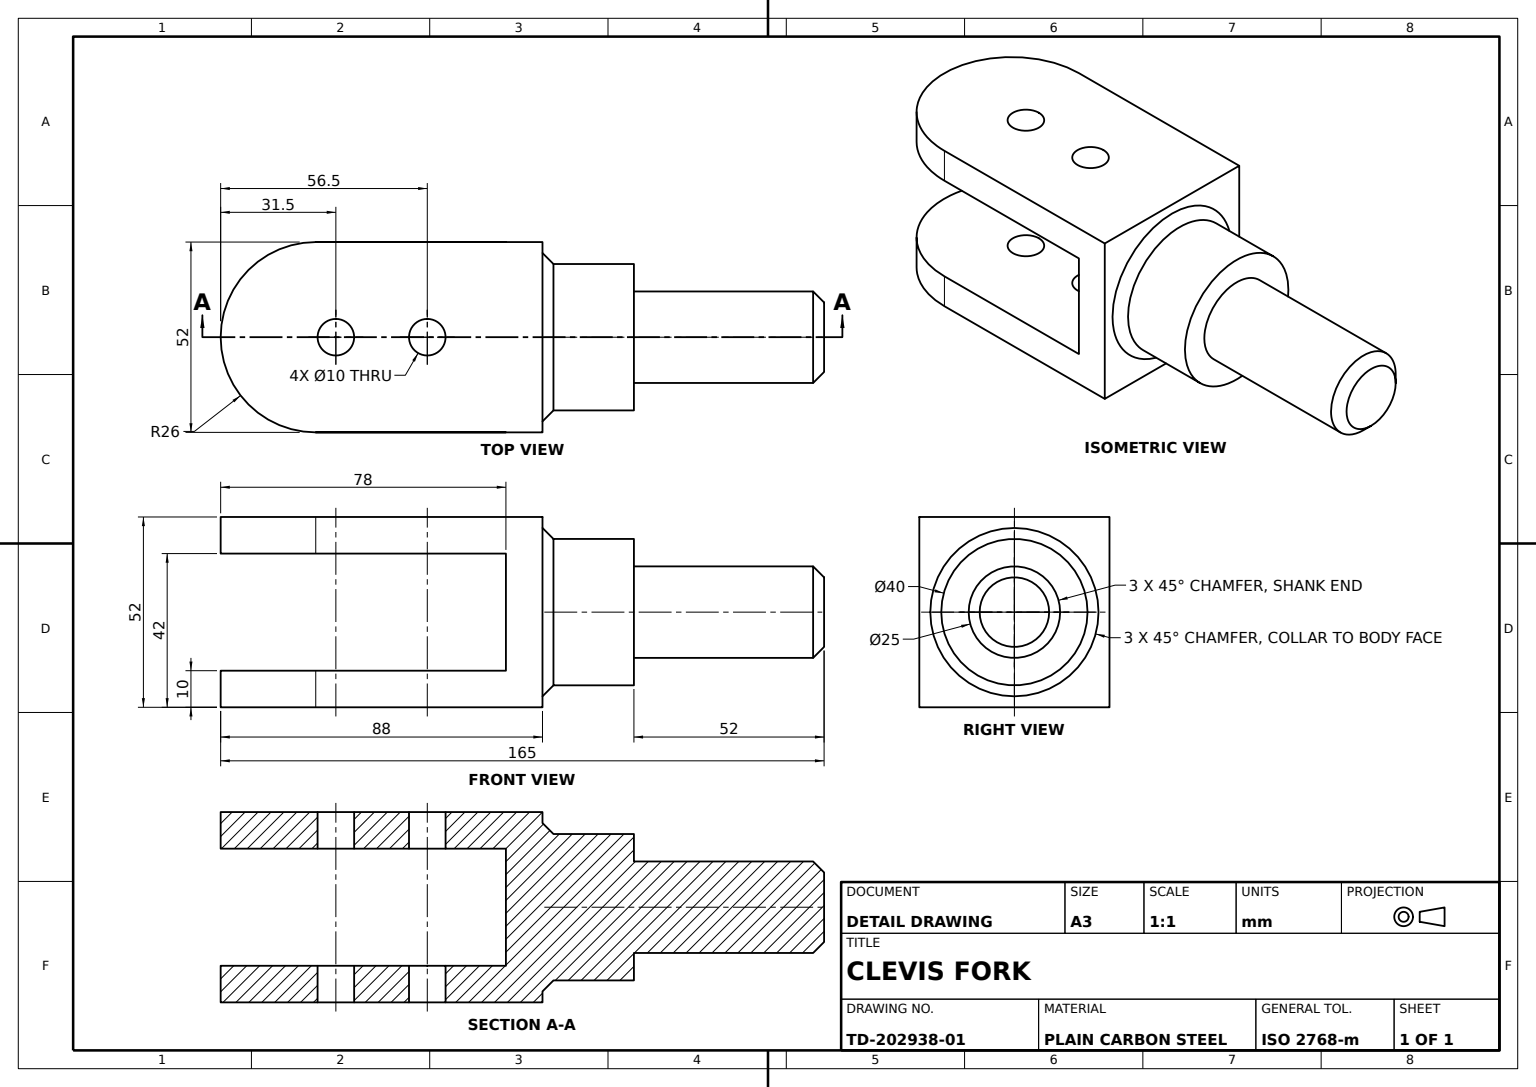
from build123d import *

# Parameters (mm, degrees)
CLEVIS_BODY_52MM_DEPTH          = 52
ARM_END_BOSS_1_DEPTH            = 10
ARM_START                       = -10
ARM_END_BOSS_2_DEPTH            = 10
FORK_START                      = -70
FORK_TRIM_CUT_DEPTH             = 70
FORK_SLOT_PROFILE_W             = 26
FORK_SLOT_PROFILE_H             = 52
FORK_SLOT_CUT_DEPTH             = 70
ARM_END_BOSS_3_DEPTH            = 10
ARM_END_BOSS_4_DEPTH            = 10
COLLAR_PROFILE_R                = 20
COLLAR_25MM_DEPTH               = 25
COLLAR_CHAMFER_3X45_SIZE        = 3
SHANK_PROFILE_R                 = 12.5
SHANK_52MM_DEPTH                = 52
SHANK_END_CHAMFER_3X45_SIZE     = 3
PIN_HOLES_PROFILE_R             = 5
PIN_HOLES_2X_THROUGH_ARMS_DEPTH = 52


with BuildPart() as part:
    # Clevis Body Profile → Clevis Body 52mm (new body)
    with BuildSketch(Plane.XY):
        Polygon((0, 0), (88, 0), (88, -10), (10, -10), (10, -42), (88, -42), (88, -52), (0, -52), align=None)
    extrude(amount=CLEVIS_BODY_52MM_DEPTH)

    # Arm End Boss 1 Profile → Arm End Boss 1 (add)
    with BuildSketch(Plane(origin=(0, 0, 0), x_dir=(1, 0, 0), z_dir=(0, 1, 0))):
        with BuildLine():
            Line((88, 0), (88, -52))
            ThreePointArc((88, -52), (114, -26), (88, 0))
        make_face()
    extrude(amount=-ARM_END_BOSS_1_DEPTH)

    # Arm End Boss 2 Profile → Arm End Boss 2 (add)
    with BuildSketch(Plane.XZ.offset(52).offset(ARM_START)):
        with BuildLine():
            Line((88, 52), (88, 0))
            ThreePointArc((88, 0), (114, 26), (88, 52))
        make_face()
    extrude(amount=ARM_END_BOSS_2_DEPTH)

    # Fork Trim Cut Profile → Fork Trim Cut (cut)
    with BuildSketch(Plane.XZ.offset(52).offset(FORK_START)):
        with BuildLine():
            Line((88, 52), (88, 0))
            ThreePointArc((88, 0), (114, 26), (88, 52))
        make_face()
    extrude(amount=FORK_TRIM_CUT_DEPTH, mode=Mode.SUBTRACT)

    # Fork Slot Profile → Fork Slot Cut (cut)
    with BuildSketch(Plane.XZ.offset(52)):
        with Locations((75, 26)):
            Rectangle(FORK_SLOT_PROFILE_W, FORK_SLOT_PROFILE_H)
    extrude(amount=-FORK_SLOT_CUT_DEPTH, mode=Mode.SUBTRACT)

    # Arm End Boss 3 Profile → Arm End Boss 3 (add)
    with BuildSketch(Plane.XZ.offset(52)):
        with BuildLine():
            Line((62, 52), (62, 0))
            ThreePointArc((62, 0), (88, 26), (62, 52))
        make_face()
    extrude(amount=-ARM_END_BOSS_3_DEPTH)

    # Arm End Boss 4 Profile → Arm End Boss 4 (add)
    with BuildSketch(Plane(origin=(0, 0, 0), x_dir=(1, 0, 0), z_dir=(0, 1, 0)).offset(ARM_START)):
        with BuildLine():
            Line((62, 0), (62, -52))
            ThreePointArc((62, -52), (88, -26), (62, 0))
        make_face()
    extrude(amount=ARM_END_BOSS_4_DEPTH)

    # Collar Profile → Collar 25mm (add)
    with BuildSketch(Plane.ZY):
        with Locations((26, -26)):
            Circle(COLLAR_PROFILE_R)
    extrude(amount=COLLAR_25MM_DEPTH)

    # Collar Chamfer 3x45
    collar_chamfer_3x45_edges = [part.edges().sort_by_distance(p)[0] for p in [
        (0, -26, 6),
    ]]
    chamfer(collar_chamfer_3x45_edges, length=COLLAR_CHAMFER_3X45_SIZE)

    # Shank Profile → Shank 52mm (add)
    with BuildSketch(Plane.ZY.offset(25)):
        with Locations(Location((26, -26, 0), (0, 0, 180))):
            Circle(SHANK_PROFILE_R)
    extrude(amount=SHANK_52MM_DEPTH)

    # Shank End Chamfer 3x45
    shank_end_chamfer_3x45_edges = [part.edges().sort_by_distance(p)[0] for p in [
        (-77, -26, 38.5),
    ]]
    chamfer(shank_end_chamfer_3x45_edges, length=SHANK_END_CHAMFER_3X45_SIZE)

    # Pin Holes Profile → Pin Holes 2x Through Arms (cut)
    with BuildSketch(Plane.XZ.offset(52)):
        with Locations(Location((31.5, 26, 0), (0, 0, 270))):
            Circle(PIN_HOLES_PROFILE_R)
        with Locations(Location((56.5, 26, 0), (0, 0, 270))):
            Circle(PIN_HOLES_PROFILE_R)
    extrude(amount=-PIN_HOLES_2X_THROUGH_ARMS_DEPTH, mode=Mode.SUBTRACT)


solid = part.part
